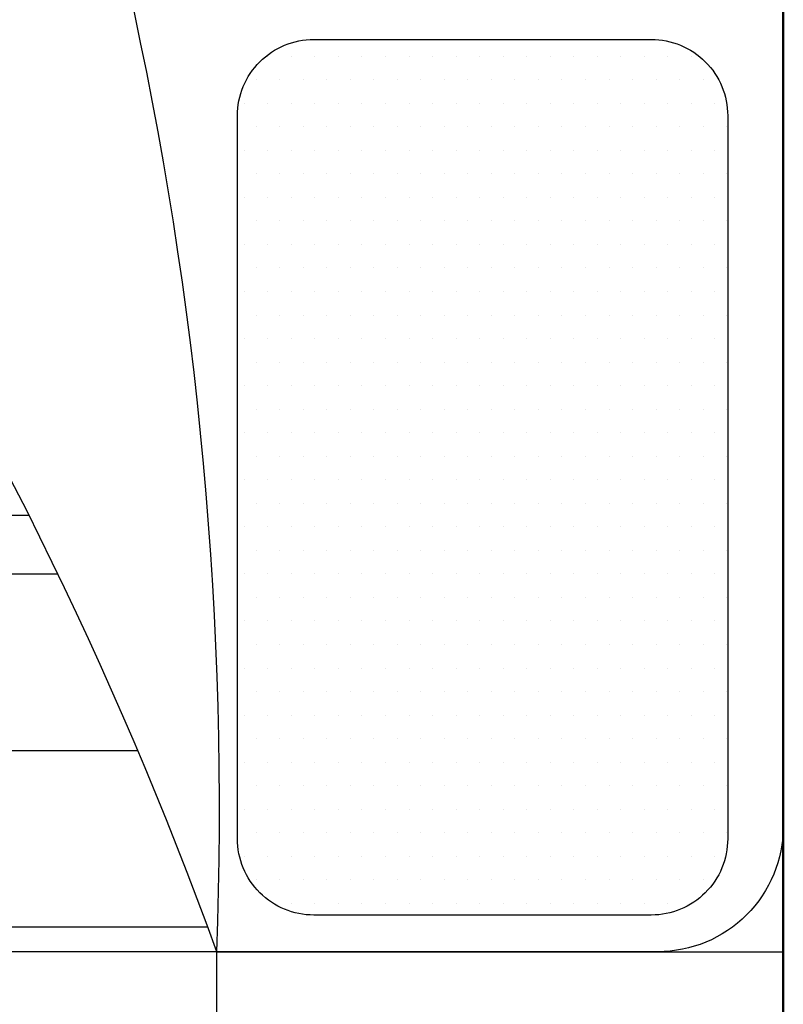
# Model space of a CAD drawing. Units: inches. Extents: x 3064 to 19385, y 846 to 15425.
# Tile 39 of 108: x 5302 to 5326, y 1028 to 1059. Entities that reach past the tile are written whole.
import ezdxf

# ---------------------------------------------------------------- set-up
doc = ezdxf.new("R2010")
doc.units = ezdxf.units.IN
doc.layers.add('A-FLOR-FIXT', color=9, linetype='Continuous', lineweight=18)
doc.layers.add('A-WALL', color=7, linetype='Continuous', lineweight=50)
doc.layers.add('BLOCK', color=6, linetype='Continuous')

# ---------------------------------------------------------------- blocks, each defined once
blk = doc.blocks.new('*X6')
at = {"color": 0}
for p, q in [((280.3125, 439.8862), (280.3125, 452.8965)), ((278.9062, 439.4824), (278.9062, 452.3385)), ((277.5, 439.4824), (277.5, 451.7019)), ((277.0312, 439.4824), (277.0312, 451.4714))]:
    blk.add_line(p, q, dxfattribs=at)
blk = doc.blocks.new('*X7')
at = {"color": 0}
for p, q in [((273.9375, 457.03125), (273.9375, 457.03125)), ((274.3125, 457.03125), (274.3125, 457.03125)), ((274.6875, 457.03125), (274.6875, 457.03125)), ((275.0625, 457.03125), (275.0625, 457.03125)), ((275.4375, 457.03125), (275.4375, 457.03125)), ((275.8125, 457.03125), (275.8125, 457.03125)), ((276.1875, 457.03125), (276.1875, 457.03125)), ((276.5625, 457.03125), (276.5625, 457.03125)), ((276.9375, 457.03125), (276.9375, 457.03125)), ((277.3125, 457.03125), (277.3125, 457.03125)), ((277.6875, 457.03125), (277.6875, 457.03125)), ((278.0625, 457.03125), (278.0625, 457.03125)), ((278.4375, 457.03125), (278.4375, 457.03125)), ((278.8125, 457.03125), (278.8125, 457.03125)), ((279.1875, 457.03125), (279.1875, 457.03125)), ((279.5625, 457.03125), (279.5625, 457.03125)), ((273.75, 456.9375), (273.75, 456.9375)), ((274.125, 456.9375), (274.125, 456.9375)), ((274.5, 456.9375), (274.5, 456.9375)), ((274.875, 456.9375), (274.875, 456.9375)), ((275.25, 456.9375), (275.25, 456.9375)), ((275.625, 456.9375), (275.625, 456.9375)), ((276, 456.9375), (276, 456.9375)), ((276.375, 456.9375), (276.375, 456.9375)), ((276.75, 456.9375), (276.75, 456.9375)), ((277.125, 456.9375), (277.125, 456.9375)), ((277.5, 456.9375), (277.5, 456.9375)), ((277.875, 456.9375), (277.875, 456.9375)), ((278.25, 456.9375), (278.25, 456.9375)), ((278.625, 456.9375), (278.625, 456.9375)), ((279, 456.9375), (279, 456.9375)), ((279.375, 456.9375), (279.375, 456.9375)), ((279.75, 456.9375), (279.75, 456.9375)), ((273.5625, 456.84375), (273.5625, 456.84375)), ((273.9375, 456.84375), (273.9375, 456.84375)), ((274.3125, 456.84375), (274.3125, 456.84375)), ((274.6875, 456.84375), (274.6875, 456.84375)), ((275.0625, 456.84375), (275.0625, 456.84375)), ((275.4375, 456.84375), (275.4375, 456.84375)), ((275.8125, 456.84375), (275.8125, 456.84375)), ((276.1875, 456.84375), (276.1875, 456.84375)), ((276.5625, 456.84375), (276.5625, 456.84375)), ((276.9375, 456.84375), (276.9375, 456.84375)), ((277.3125, 456.84375), (277.3125, 456.84375)), ((277.6875, 456.84375), (277.6875, 456.84375)), ((278.0625, 456.84375), (278.0625, 456.84375)), ((278.4375, 456.84375), (278.4375, 456.84375)), ((278.8125, 456.84375), (278.8125, 456.84375)), ((279.1875, 456.84375), (279.1875, 456.84375)), ((279.5625, 456.84375), (279.5625, 456.84375)), ((279.9375, 456.84375), (279.9375, 456.84375)), ((273.375, 456.75), (273.375, 456.75)), ((273.75, 456.75), (273.75, 456.75)), ((274.125, 456.75), (274.125, 456.75)), ((274.5, 456.75), (274.5, 456.75)), ((274.875, 456.75), (274.875, 456.75)), ((275.25, 456.75), (275.25, 456.75)), ((275.625, 456.75), (275.625, 456.75)), ((276, 456.75), (276, 456.75)), ((276.375, 456.75), (276.375, 456.75)), ((276.75, 456.75), (276.75, 456.75)), ((277.125, 456.75), (277.125, 456.75)), ((277.5, 456.75), (277.5, 456.75)), ((277.875, 456.75), (277.875, 456.75)), ((278.25, 456.75), (278.25, 456.75)), ((278.625, 456.75), (278.625, 456.75)), ((279, 456.75), (279, 456.75)), ((279.375, 456.75), (279.375, 456.75)), ((279.75, 456.75), (279.75, 456.75)), ((280.125, 456.75), (280.125, 456.75)), ((273.5625, 456.65625), (273.5625, 456.65625)), ((273.9375, 456.65625), (273.9375, 456.65625)), ((274.3125, 456.65625), (274.3125, 456.65625)), ((274.6875, 456.65625), (274.6875, 456.65625)), ((275.0625, 456.65625), (275.0625, 456.65625)), ((275.4375, 456.65625), (275.4375, 456.65625)), ((275.8125, 456.65625), (275.8125, 456.65625)), ((276.1875, 456.65625), (276.1875, 456.65625)), ((276.5625, 456.65625), (276.5625, 456.65625)), ((276.9375, 456.65625), (276.9375, 456.65625)), ((277.3125, 456.65625), (277.3125, 456.65625)), ((277.6875, 456.65625), (277.6875, 456.65625)), ((278.0625, 456.65625), (278.0625, 456.65625)), ((278.4375, 456.65625), (278.4375, 456.65625)), ((278.8125, 456.65625), (278.8125, 456.65625)), ((279.1875, 456.65625), (279.1875, 456.65625)), ((279.5625, 456.65625), (279.5625, 456.65625)), ((279.9375, 456.65625), (279.9375, 456.65625)), ((273.375, 456.5625), (273.375, 456.5625)), ((273.75, 456.5625), (273.75, 456.5625)), ((274.125, 456.5625), (274.125, 456.5625)), ((274.5, 456.5625), (274.5, 456.5625)), ((274.875, 456.5625), (274.875, 456.5625)), ((275.25, 456.5625), (275.25, 456.5625)), ((275.625, 456.5625), (275.625, 456.5625)), ((276, 456.5625), (276, 456.5625)), ((276.375, 456.5625), (276.375, 456.5625)), ((276.75, 456.5625), (276.75, 456.5625)), ((277.125, 456.5625), (277.125, 456.5625)), ((277.5, 456.5625), (277.5, 456.5625)), ((277.875, 456.5625), (277.875, 456.5625)), ((278.25, 456.5625), (278.25, 456.5625)), ((278.625, 456.5625), (278.625, 456.5625)), ((279, 456.5625), (279, 456.5625)), ((279.375, 456.5625), (279.375, 456.5625)), ((279.75, 456.5625), (279.75, 456.5625)), ((280.125, 456.5625), (280.125, 456.5625)), ((273.5625, 456.46875), (273.5625, 456.46875)), ((273.9375, 456.46875), (273.9375, 456.46875)), ((274.3125, 456.46875), (274.3125, 456.46875)), ((274.6875, 456.46875), (274.6875, 456.46875)), ((275.0625, 456.46875), (275.0625, 456.46875)), ((275.4375, 456.46875), (275.4375, 456.46875)), ((275.8125, 456.46875), (275.8125, 456.46875)), ((276.1875, 456.46875), (276.1875, 456.46875)), ((276.5625, 456.46875), (276.5625, 456.46875)), ((276.9375, 456.46875), (276.9375, 456.46875)), ((277.3125, 456.46875), (277.3125, 456.46875)), ((277.6875, 456.46875), (277.6875, 456.46875)), ((278.0625, 456.46875), (278.0625, 456.46875)), ((278.4375, 456.46875), (278.4375, 456.46875)), ((278.8125, 456.46875), (278.8125, 456.46875)), ((279.1875, 456.46875), (279.1875, 456.46875)), ((279.5625, 456.46875), (279.5625, 456.46875)), ((279.9375, 456.46875), (279.9375, 456.46875)), ((273.375, 456.375), (273.375, 456.375)), ((273.75, 456.375), (273.75, 456.375)), ((274.125, 456.375), (274.125, 456.375)), ((274.5, 456.375), (274.5, 456.375)), ((274.875, 456.375), (274.875, 456.375)), ((275.25, 456.375), (275.25, 456.375)), ((275.625, 456.375), (275.625, 456.375)), ((276, 456.375), (276, 456.375)), ((276.375, 456.375), (276.375, 456.375)), ((276.75, 456.375), (276.75, 456.375)), ((277.125, 456.375), (277.125, 456.375)), ((277.5, 456.375), (277.5, 456.375)), ((277.875, 456.375), (277.875, 456.375)), ((278.25, 456.375), (278.25, 456.375)), ((278.625, 456.375), (278.625, 456.375)), ((279, 456.375), (279, 456.375)), ((279.375, 456.375), (279.375, 456.375)), ((279.75, 456.375), (279.75, 456.375)), ((280.125, 456.375), (280.125, 456.375)), ((273.5625, 456.28125), (273.5625, 456.28125)), ((273.9375, 456.28125), (273.9375, 456.28125)), ((274.3125, 456.28125), (274.3125, 456.28125)), ((274.6875, 456.28125), (274.6875, 456.28125)), ((275.0625, 456.28125), (275.0625, 456.28125)), ((275.4375, 456.28125), (275.4375, 456.28125)), ((275.8125, 456.28125), (275.8125, 456.28125)), ((276.1875, 456.28125), (276.1875, 456.28125)), ((276.5625, 456.28125), (276.5625, 456.28125)), ((276.9375, 456.28125), (276.9375, 456.28125)), ((277.3125, 456.28125), (277.3125, 456.28125)), ((277.6875, 456.28125), (277.6875, 456.28125)), ((278.0625, 456.28125), (278.0625, 456.28125)), ((278.4375, 456.28125), (278.4375, 456.28125)), ((278.8125, 456.28125), (278.8125, 456.28125)), ((279.1875, 456.28125), (279.1875, 456.28125)), ((279.5625, 456.28125), (279.5625, 456.28125)), ((279.9375, 456.28125), (279.9375, 456.28125)), ((273.375, 456.1875), (273.375, 456.1875)), ((273.75, 456.1875), (273.75, 456.1875)), ((274.125, 456.1875), (274.125, 456.1875)), ((274.5, 456.1875), (274.5, 456.1875)), ((274.875, 456.1875), (274.875, 456.1875)), ((275.25, 456.1875), (275.25, 456.1875)), ((275.625, 456.1875), (275.625, 456.1875)), ((276, 456.1875), (276, 456.1875)), ((276.375, 456.1875), (276.375, 456.1875)), ((276.75, 456.1875), (276.75, 456.1875)), ((277.125, 456.1875), (277.125, 456.1875)), ((277.5, 456.1875), (277.5, 456.1875)), ((277.875, 456.1875), (277.875, 456.1875)), ((278.25, 456.1875), (278.25, 456.1875)), ((278.625, 456.1875), (278.625, 456.1875)), ((279, 456.1875), (279, 456.1875)), ((279.375, 456.1875), (279.375, 456.1875)), ((279.75, 456.1875), (279.75, 456.1875)), ((280.125, 456.1875), (280.125, 456.1875)), ((273.5625, 456.09375), (273.5625, 456.09375)), ((273.9375, 456.09375), (273.9375, 456.09375)), ((274.3125, 456.09375), (274.3125, 456.09375)), ((274.6875, 456.09375), (274.6875, 456.09375)), ((275.0625, 456.09375), (275.0625, 456.09375)), ((275.4375, 456.09375), (275.4375, 456.09375)), ((275.8125, 456.09375), (275.8125, 456.09375)), ((276.1875, 456.09375), (276.1875, 456.09375)), ((276.5625, 456.09375), (276.5625, 456.09375)), ((276.9375, 456.09375), (276.9375, 456.09375)), ((277.3125, 456.09375), (277.3125, 456.09375)), ((277.6875, 456.09375), (277.6875, 456.09375)), ((278.0625, 456.09375), (278.0625, 456.09375)), ((278.4375, 456.09375), (278.4375, 456.09375)), ((278.8125, 456.09375), (278.8125, 456.09375)), ((279.1875, 456.09375), (279.1875, 456.09375)), ((279.5625, 456.09375), (279.5625, 456.09375)), ((279.9375, 456.09375), (279.9375, 456.09375)), ((273.375, 456), (273.375, 456)), ((273.75, 456), (273.75, 456)), ((274.125, 456), (274.125, 456)), ((274.5, 456), (274.5, 456)), ((274.875, 456), (274.875, 456)), ((275.25, 456), (275.25, 456)), ((275.625, 456), (275.625, 456)), ((276, 456), (276, 456)), ((276.375, 456), (276.375, 456)), ((276.75, 456), (276.75, 456)), ((277.125, 456), (277.125, 456)), ((277.5, 456), (277.5, 456)), ((277.875, 456), (277.875, 456)), ((278.25, 456), (278.25, 456)), ((278.625, 456), (278.625, 456)), ((279, 456), (279, 456)), ((279.375, 456), (279.375, 456)), ((279.75, 456), (279.75, 456)), ((280.125, 456), (280.125, 456)), ((273.5625, 455.90625), (273.5625, 455.90625)), ((273.9375, 455.90625), (273.9375, 455.90625)), ((274.3125, 455.90625), (274.3125, 455.90625)), ((274.6875, 455.90625), (274.6875, 455.90625)), ((275.0625, 455.90625), (275.0625, 455.90625)), ((275.4375, 455.90625), (275.4375, 455.90625)), ((275.8125, 455.90625), (275.8125, 455.90625)), ((276.1875, 455.90625), (276.1875, 455.90625)), ((276.5625, 455.90625), (276.5625, 455.90625)), ((276.9375, 455.90625), (276.9375, 455.90625)), ((277.3125, 455.90625), (277.3125, 455.90625)), ((277.6875, 455.90625), (277.6875, 455.90625)), ((278.0625, 455.90625), (278.0625, 455.90625)), ((278.4375, 455.90625), (278.4375, 455.90625)), ((278.8125, 455.90625), (278.8125, 455.90625)), ((279.1875, 455.90625), (279.1875, 455.90625)), ((279.5625, 455.90625), (279.5625, 455.90625)), ((279.9375, 455.90625), (279.9375, 455.90625)), ((273.375, 455.8125), (273.375, 455.8125)), ((273.75, 455.8125), (273.75, 455.8125)), ((274.125, 455.8125), (274.125, 455.8125)), ((274.5, 455.8125), (274.5, 455.8125)), ((274.875, 455.8125), (274.875, 455.8125)), ((275.25, 455.8125), (275.25, 455.8125)), ((275.625, 455.8125), (275.625, 455.8125)), ((276, 455.8125), (276, 455.8125)), ((276.375, 455.8125), (276.375, 455.8125)), ((276.75, 455.8125), (276.75, 455.8125)), ((277.125, 455.8125), (277.125, 455.8125)), ((277.5, 455.8125), (277.5, 455.8125)), ((277.875, 455.8125), (277.875, 455.8125)), ((278.25, 455.8125), (278.25, 455.8125)), ((278.625, 455.8125), (278.625, 455.8125)), ((279, 455.8125), (279, 455.8125)), ((279.375, 455.8125), (279.375, 455.8125)), ((279.75, 455.8125), (279.75, 455.8125)), ((280.125, 455.8125), (280.125, 455.8125)), ((273.5625, 455.71875), (273.5625, 455.71875)), ((273.9375, 455.71875), (273.9375, 455.71875)), ((274.3125, 455.71875), (274.3125, 455.71875)), ((274.6875, 455.71875), (274.6875, 455.71875)), ((275.0625, 455.71875), (275.0625, 455.71875)), ((275.4375, 455.71875), (275.4375, 455.71875)), ((275.8125, 455.71875), (275.8125, 455.71875)), ((276.1875, 455.71875), (276.1875, 455.71875)), ((276.5625, 455.71875), (276.5625, 455.71875)), ((276.9375, 455.71875), (276.9375, 455.71875)), ((277.3125, 455.71875), (277.3125, 455.71875)), ((277.6875, 455.71875), (277.6875, 455.71875)), ((278.0625, 455.71875), (278.0625, 455.71875)), ((278.4375, 455.71875), (278.4375, 455.71875)), ((278.8125, 455.71875), (278.8125, 455.71875)), ((279.1875, 455.71875), (279.1875, 455.71875)), ((279.5625, 455.71875), (279.5625, 455.71875)), ((279.9375, 455.71875), (279.9375, 455.71875)), ((273.375, 455.625), (273.375, 455.625)), ((273.75, 455.625), (273.75, 455.625)), ((274.125, 455.625), (274.125, 455.625)), ((274.5, 455.625), (274.5, 455.625)), ((274.875, 455.625), (274.875, 455.625)), ((275.25, 455.625), (275.25, 455.625)), ((275.625, 455.625), (275.625, 455.625)), ((276, 455.625), (276, 455.625)), ((276.375, 455.625), (276.375, 455.625)), ((276.75, 455.625), (276.75, 455.625)), ((277.125, 455.625), (277.125, 455.625)), ((277.5, 455.625), (277.5, 455.625)), ((277.875, 455.625), (277.875, 455.625)), ((278.25, 455.625), (278.25, 455.625)), ((278.625, 455.625), (278.625, 455.625)), ((279, 455.625), (279, 455.625)), ((279.375, 455.625), (279.375, 455.625)), ((279.75, 455.625), (279.75, 455.625)), ((280.125, 455.625), (280.125, 455.625)), ((273.5625, 455.53125), (273.5625, 455.53125)), ((273.9375, 455.53125), (273.9375, 455.53125)), ((274.3125, 455.53125), (274.3125, 455.53125)), ((274.6875, 455.53125), (274.6875, 455.53125)), ((275.0625, 455.53125), (275.0625, 455.53125)), ((275.4375, 455.53125), (275.4375, 455.53125)), ((275.8125, 455.53125), (275.8125, 455.53125)), ((276.1875, 455.53125), (276.1875, 455.53125)), ((276.5625, 455.53125), (276.5625, 455.53125)), ((276.9375, 455.53125), (276.9375, 455.53125)), ((277.3125, 455.53125), (277.3125, 455.53125)), ((277.6875, 455.53125), (277.6875, 455.53125)), ((278.0625, 455.53125), (278.0625, 455.53125)), ((278.4375, 455.53125), (278.4375, 455.53125)), ((278.8125, 455.53125), (278.8125, 455.53125)), ((279.1875, 455.53125), (279.1875, 455.53125)), ((279.5625, 455.53125), (279.5625, 455.53125)), ((279.9375, 455.53125), (279.9375, 455.53125)), ((273.375, 455.4375), (273.375, 455.4375)), ((273.75, 455.4375), (273.75, 455.4375)), ((274.125, 455.4375), (274.125, 455.4375)), ((274.5, 455.4375), (274.5, 455.4375)), ((274.875, 455.4375), (274.875, 455.4375)), ((275.25, 455.4375), (275.25, 455.4375)), ((275.625, 455.4375), (275.625, 455.4375)), ((276, 455.4375), (276, 455.4375)), ((276.375, 455.4375), (276.375, 455.4375)), ((276.75, 455.4375), (276.75, 455.4375)), ((277.125, 455.4375), (277.125, 455.4375)), ((277.5, 455.4375), (277.5, 455.4375)), ((277.875, 455.4375), (277.875, 455.4375)), ((278.25, 455.4375), (278.25, 455.4375)), ((278.625, 455.4375), (278.625, 455.4375)), ((279, 455.4375), (279, 455.4375)), ((279.375, 455.4375), (279.375, 455.4375)), ((279.75, 455.4375), (279.75, 455.4375)), ((280.125, 455.4375), (280.125, 455.4375)), ((273.5625, 455.34375), (273.5625, 455.34375)), ((273.9375, 455.34375), (273.9375, 455.34375)), ((274.3125, 455.34375), (274.3125, 455.34375)), ((274.6875, 455.34375), (274.6875, 455.34375)), ((275.0625, 455.34375), (275.0625, 455.34375)), ((275.4375, 455.34375), (275.4375, 455.34375)), ((275.8125, 455.34375), (275.8125, 455.34375)), ((276.1875, 455.34375), (276.1875, 455.34375)), ((276.5625, 455.34375), (276.5625, 455.34375)), ((276.9375, 455.34375), (276.9375, 455.34375)), ((277.3125, 455.34375), (277.3125, 455.34375)), ((277.6875, 455.34375), (277.6875, 455.34375)), ((278.0625, 455.34375), (278.0625, 455.34375)), ((278.4375, 455.34375), (278.4375, 455.34375)), ((278.8125, 455.34375), (278.8125, 455.34375)), ((279.1875, 455.34375), (279.1875, 455.34375)), ((279.5625, 455.34375), (279.5625, 455.34375)), ((279.9375, 455.34375), (279.9375, 455.34375)), ((273.375, 455.25), (273.375, 455.25)), ((273.75, 455.25), (273.75, 455.25)), ((274.125, 455.25), (274.125, 455.25)), ((274.5, 455.25), (274.5, 455.25)), ((274.875, 455.25), (274.875, 455.25)), ((275.25, 455.25), (275.25, 455.25)), ((275.625, 455.25), (275.625, 455.25)), ((276, 455.25), (276, 455.25)), ((276.375, 455.25), (276.375, 455.25)), ((276.75, 455.25), (276.75, 455.25)), ((277.125, 455.25), (277.125, 455.25)), ((277.5, 455.25), (277.5, 455.25)), ((277.875, 455.25), (277.875, 455.25)), ((278.25, 455.25), (278.25, 455.25)), ((278.625, 455.25), (278.625, 455.25)), ((279, 455.25), (279, 455.25)), ((279.375, 455.25), (279.375, 455.25)), ((279.75, 455.25), (279.75, 455.25)), ((280.125, 455.25), (280.125, 455.25)), ((273.5625, 455.15625), (273.5625, 455.15625)), ((273.9375, 455.15625), (273.9375, 455.15625)), ((274.3125, 455.15625), (274.3125, 455.15625)), ((274.6875, 455.15625), (274.6875, 455.15625)), ((275.0625, 455.15625), (275.0625, 455.15625)), ((275.4375, 455.15625), (275.4375, 455.15625)), ((275.8125, 455.15625), (275.8125, 455.15625)), ((276.1875, 455.15625), (276.1875, 455.15625)), ((276.5625, 455.15625), (276.5625, 455.15625)), ((276.9375, 455.15625), (276.9375, 455.15625)), ((277.3125, 455.15625), (277.3125, 455.15625)), ((277.6875, 455.15625), (277.6875, 455.15625)), ((278.0625, 455.15625), (278.0625, 455.15625)), ((278.4375, 455.15625), (278.4375, 455.15625)), ((278.8125, 455.15625), (278.8125, 455.15625)), ((279.1875, 455.15625), (279.1875, 455.15625)), ((279.5625, 455.15625), (279.5625, 455.15625)), ((279.9375, 455.15625), (279.9375, 455.15625)), ((273.375, 455.0625), (273.375, 455.0625)), ((273.75, 455.0625), (273.75, 455.0625)), ((274.125, 455.0625), (274.125, 455.0625)), ((274.5, 455.0625), (274.5, 455.0625)), ((274.875, 455.0625), (274.875, 455.0625)), ((275.25, 455.0625), (275.25, 455.0625)), ((275.625, 455.0625), (275.625, 455.0625)), ((276, 455.0625), (276, 455.0625)), ((276.375, 455.0625), (276.375, 455.0625)), ((276.75, 455.0625), (276.75, 455.0625)), ((277.125, 455.0625), (277.125, 455.0625)), ((277.5, 455.0625), (277.5, 455.0625)), ((277.875, 455.0625), (277.875, 455.0625)), ((278.25, 455.0625), (278.25, 455.0625)), ((278.625, 455.0625), (278.625, 455.0625)), ((279, 455.0625), (279, 455.0625)), ((279.375, 455.0625), (279.375, 455.0625)), ((279.75, 455.0625), (279.75, 455.0625)), ((280.125, 455.0625), (280.125, 455.0625)), ((273.5625, 454.96875), (273.5625, 454.96875)), ((273.9375, 454.96875), (273.9375, 454.96875)), ((274.3125, 454.96875), (274.3125, 454.96875)), ((274.6875, 454.96875), (274.6875, 454.96875)), ((275.0625, 454.96875), (275.0625, 454.96875)), ((275.4375, 454.96875), (275.4375, 454.96875)), ((275.8125, 454.96875), (275.8125, 454.96875)), ((276.1875, 454.96875), (276.1875, 454.96875)), ((276.5625, 454.96875), (276.5625, 454.96875)), ((276.9375, 454.96875), (276.9375, 454.96875)), ((277.3125, 454.96875), (277.3125, 454.96875)), ((277.6875, 454.96875), (277.6875, 454.96875)), ((278.0625, 454.96875), (278.0625, 454.96875)), ((278.4375, 454.96875), (278.4375, 454.96875)), ((278.8125, 454.96875), (278.8125, 454.96875)), ((279.1875, 454.96875), (279.1875, 454.96875)), ((279.5625, 454.96875), (279.5625, 454.96875)), ((279.9375, 454.96875), (279.9375, 454.96875)), ((273.375, 454.875), (273.375, 454.875)), ((273.75, 454.875), (273.75, 454.875)), ((274.125, 454.875), (274.125, 454.875)), ((274.5, 454.875), (274.5, 454.875)), ((274.875, 454.875), (274.875, 454.875)), ((275.25, 454.875), (275.25, 454.875)), ((275.625, 454.875), (275.625, 454.875)), ((276, 454.875), (276, 454.875)), ((276.375, 454.875), (276.375, 454.875)), ((276.75, 454.875), (276.75, 454.875)), ((277.125, 454.875), (277.125, 454.875)), ((277.5, 454.875), (277.5, 454.875)), ((277.875, 454.875), (277.875, 454.875)), ((278.25, 454.875), (278.25, 454.875)), ((278.625, 454.875), (278.625, 454.875)), ((279, 454.875), (279, 454.875)), ((279.375, 454.875), (279.375, 454.875)), ((279.75, 454.875), (279.75, 454.875)), ((280.125, 454.875), (280.125, 454.875)), ((273.5625, 454.78125), (273.5625, 454.78125)), ((273.9375, 454.78125), (273.9375, 454.78125)), ((274.3125, 454.78125), (274.3125, 454.78125)), ((274.6875, 454.78125), (274.6875, 454.78125)), ((275.0625, 454.78125), (275.0625, 454.78125)), ((275.4375, 454.78125), (275.4375, 454.78125)), ((275.8125, 454.78125), (275.8125, 454.78125)), ((276.1875, 454.78125), (276.1875, 454.78125)), ((276.5625, 454.78125), (276.5625, 454.78125)), ((276.9375, 454.78125), (276.9375, 454.78125)), ((277.3125, 454.78125), (277.3125, 454.78125)), ((277.6875, 454.78125), (277.6875, 454.78125)), ((278.0625, 454.78125), (278.0625, 454.78125)), ((278.4375, 454.78125), (278.4375, 454.78125)), ((278.8125, 454.78125), (278.8125, 454.78125)), ((279.1875, 454.78125), (279.1875, 454.78125)), ((279.5625, 454.78125), (279.5625, 454.78125)), ((279.9375, 454.78125), (279.9375, 454.78125)), ((273.375, 454.6875), (273.375, 454.6875)), ((273.75, 454.6875), (273.75, 454.6875)), ((274.125, 454.6875), (274.125, 454.6875)), ((274.5, 454.6875), (274.5, 454.6875)), ((274.875, 454.6875), (274.875, 454.6875)), ((275.25, 454.6875), (275.25, 454.6875)), ((275.625, 454.6875), (275.625, 454.6875)), ((276, 454.6875), (276, 454.6875)), ((276.375, 454.6875), (276.375, 454.6875)), ((276.75, 454.6875), (276.75, 454.6875)), ((277.125, 454.6875), (277.125, 454.6875)), ((277.5, 454.6875), (277.5, 454.6875)), ((277.875, 454.6875), (277.875, 454.6875)), ((278.25, 454.6875), (278.25, 454.6875)), ((278.625, 454.6875), (278.625, 454.6875)), ((279, 454.6875), (279, 454.6875)), ((279.375, 454.6875), (279.375, 454.6875)), ((279.75, 454.6875), (279.75, 454.6875)), ((280.125, 454.6875), (280.125, 454.6875)), ((273.5625, 454.59375), (273.5625, 454.59375)), ((273.9375, 454.59375), (273.9375, 454.59375)), ((274.3125, 454.59375), (274.3125, 454.59375)), ((274.6875, 454.59375), (274.6875, 454.59375)), ((275.0625, 454.59375), (275.0625, 454.59375)), ((275.4375, 454.59375), (275.4375, 454.59375)), ((275.8125, 454.59375), (275.8125, 454.59375)), ((276.1875, 454.59375), (276.1875, 454.59375)), ((276.5625, 454.59375), (276.5625, 454.59375)), ((276.9375, 454.59375), (276.9375, 454.59375)), ((277.3125, 454.59375), (277.3125, 454.59375)), ((277.6875, 454.59375), (277.6875, 454.59375)), ((278.0625, 454.59375), (278.0625, 454.59375)), ((278.4375, 454.59375), (278.4375, 454.59375)), ((278.8125, 454.59375), (278.8125, 454.59375)), ((279.1875, 454.59375), (279.1875, 454.59375)), ((279.5625, 454.59375), (279.5625, 454.59375)), ((279.9375, 454.59375), (279.9375, 454.59375)), ((273.375, 454.5), (273.375, 454.5)), ((273.75, 454.5), (273.75, 454.5)), ((274.125, 454.5), (274.125, 454.5)), ((274.5, 454.5), (274.5, 454.5)), ((274.875, 454.5), (274.875, 454.5)), ((275.25, 454.5), (275.25, 454.5)), ((275.625, 454.5), (275.625, 454.5)), ((276, 454.5), (276, 454.5)), ((276.375, 454.5), (276.375, 454.5)), ((276.75, 454.5), (276.75, 454.5)), ((277.125, 454.5), (277.125, 454.5)), ((277.5, 454.5), (277.5, 454.5)), ((277.875, 454.5), (277.875, 454.5)), ((278.25, 454.5), (278.25, 454.5)), ((278.625, 454.5), (278.625, 454.5)), ((279, 454.5), (279, 454.5)), ((279.375, 454.5), (279.375, 454.5)), ((279.75, 454.5), (279.75, 454.5)), ((280.125, 454.5), (280.125, 454.5)), ((273.5625, 454.40625), (273.5625, 454.40625)), ((273.9375, 454.40625), (273.9375, 454.40625)), ((274.3125, 454.40625), (274.3125, 454.40625)), ((274.6875, 454.40625), (274.6875, 454.40625)), ((275.0625, 454.40625), (275.0625, 454.40625)), ((275.4375, 454.40625), (275.4375, 454.40625)), ((275.8125, 454.40625), (275.8125, 454.40625)), ((276.1875, 454.40625), (276.1875, 454.40625)), ((276.5625, 454.40625), (276.5625, 454.40625)), ((276.9375, 454.40625), (276.9375, 454.40625)), ((277.3125, 454.40625), (277.3125, 454.40625)), ((277.6875, 454.40625), (277.6875, 454.40625)), ((278.0625, 454.40625), (278.0625, 454.40625)), ((278.4375, 454.40625), (278.4375, 454.40625)), ((278.8125, 454.40625), (278.8125, 454.40625)), ((279.1875, 454.40625), (279.1875, 454.40625)), ((279.5625, 454.40625), (279.5625, 454.40625)), ((279.9375, 454.40625), (279.9375, 454.40625)), ((273.375, 454.3125), (273.375, 454.3125)), ((273.75, 454.3125), (273.75, 454.3125)), ((274.125, 454.3125), (274.125, 454.3125)), ((274.5, 454.3125), (274.5, 454.3125)), ((274.875, 454.3125), (274.875, 454.3125)), ((275.25, 454.3125), (275.25, 454.3125)), ((275.625, 454.3125), (275.625, 454.3125)), ((276, 454.3125), (276, 454.3125)), ((276.375, 454.3125), (276.375, 454.3125)), ((276.75, 454.3125), (276.75, 454.3125)), ((277.125, 454.3125), (277.125, 454.3125)), ((277.5, 454.3125), (277.5, 454.3125)), ((277.875, 454.3125), (277.875, 454.3125)), ((278.25, 454.3125), (278.25, 454.3125)), ((278.625, 454.3125), (278.625, 454.3125)), ((279, 454.3125), (279, 454.3125)), ((279.375, 454.3125), (279.375, 454.3125)), ((279.75, 454.3125), (279.75, 454.3125)), ((280.125, 454.3125), (280.125, 454.3125)), ((273.5625, 454.21875), (273.5625, 454.21875)), ((273.9375, 454.21875), (273.9375, 454.21875)), ((274.3125, 454.21875), (274.3125, 454.21875)), ((274.6875, 454.21875), (274.6875, 454.21875)), ((275.0625, 454.21875), (275.0625, 454.21875)), ((275.4375, 454.21875), (275.4375, 454.21875)), ((275.8125, 454.21875), (275.8125, 454.21875)), ((276.1875, 454.21875), (276.1875, 454.21875)), ((276.5625, 454.21875), (276.5625, 454.21875)), ((276.9375, 454.21875), (276.9375, 454.21875)), ((277.3125, 454.21875), (277.3125, 454.21875)), ((277.6875, 454.21875), (277.6875, 454.21875)), ((278.0625, 454.21875), (278.0625, 454.21875)), ((278.4375, 454.21875), (278.4375, 454.21875)), ((278.8125, 454.21875), (278.8125, 454.21875)), ((279.1875, 454.21875), (279.1875, 454.21875)), ((279.5625, 454.21875), (279.5625, 454.21875)), ((279.9375, 454.21875), (279.9375, 454.21875)), ((273.375, 454.125), (273.375, 454.125)), ((273.75, 454.125), (273.75, 454.125)), ((274.125, 454.125), (274.125, 454.125)), ((274.5, 454.125), (274.5, 454.125)), ((274.875, 454.125), (274.875, 454.125)), ((275.25, 454.125), (275.25, 454.125)), ((275.625, 454.125), (275.625, 454.125)), ((276, 454.125), (276, 454.125)), ((276.375, 454.125), (276.375, 454.125)), ((276.75, 454.125), (276.75, 454.125)), ((277.125, 454.125), (277.125, 454.125)), ((277.5, 454.125), (277.5, 454.125)), ((277.875, 454.125), (277.875, 454.125)), ((278.25, 454.125), (278.25, 454.125)), ((278.625, 454.125), (278.625, 454.125)), ((279, 454.125), (279, 454.125)), ((279.375, 454.125), (279.375, 454.125)), ((279.75, 454.125), (279.75, 454.125)), ((280.125, 454.125), (280.125, 454.125)), ((273.5625, 454.03125), (273.5625, 454.03125)), ((273.9375, 454.03125), (273.9375, 454.03125)), ((274.3125, 454.03125), (274.3125, 454.03125)), ((274.6875, 454.03125), (274.6875, 454.03125)), ((275.0625, 454.03125), (275.0625, 454.03125)), ((275.4375, 454.03125), (275.4375, 454.03125)), ((275.8125, 454.03125), (275.8125, 454.03125)), ((276.1875, 454.03125), (276.1875, 454.03125)), ((276.5625, 454.03125), (276.5625, 454.03125)), ((276.9375, 454.03125), (276.9375, 454.03125)), ((277.3125, 454.03125), (277.3125, 454.03125)), ((277.6875, 454.03125), (277.6875, 454.03125)), ((278.0625, 454.03125), (278.0625, 454.03125)), ((278.4375, 454.03125), (278.4375, 454.03125)), ((278.8125, 454.03125), (278.8125, 454.03125)), ((279.1875, 454.03125), (279.1875, 454.03125)), ((279.5625, 454.03125), (279.5625, 454.03125)), ((279.9375, 454.03125), (279.9375, 454.03125)), ((273.375, 453.9375), (273.375, 453.9375)), ((273.75, 453.9375), (273.75, 453.9375)), ((274.125, 453.9375), (274.125, 453.9375)), ((274.5, 453.9375), (274.5, 453.9375)), ((274.875, 453.9375), (274.875, 453.9375)), ((275.25, 453.9375), (275.25, 453.9375)), ((275.625, 453.9375), (275.625, 453.9375)), ((276, 453.9375), (276, 453.9375)), ((276.375, 453.9375), (276.375, 453.9375)), ((276.75, 453.9375), (276.75, 453.9375)), ((277.125, 453.9375), (277.125, 453.9375)), ((277.5, 453.9375), (277.5, 453.9375)), ((277.875, 453.9375), (277.875, 453.9375)), ((278.25, 453.9375), (278.25, 453.9375)), ((278.625, 453.9375), (278.625, 453.9375)), ((279, 453.9375), (279, 453.9375)), ((279.375, 453.9375), (279.375, 453.9375)), ((279.75, 453.9375), (279.75, 453.9375)), ((280.125, 453.9375), (280.125, 453.9375)), ((273.5625, 453.84375), (273.5625, 453.84375)), ((273.9375, 453.84375), (273.9375, 453.84375)), ((274.3125, 453.84375), (274.3125, 453.84375)), ((274.6875, 453.84375), (274.6875, 453.84375)), ((275.0625, 453.84375), (275.0625, 453.84375)), ((275.4375, 453.84375), (275.4375, 453.84375)), ((275.8125, 453.84375), (275.8125, 453.84375)), ((276.1875, 453.84375), (276.1875, 453.84375)), ((276.5625, 453.84375), (276.5625, 453.84375)), ((276.9375, 453.84375), (276.9375, 453.84375)), ((277.3125, 453.84375), (277.3125, 453.84375)), ((277.6875, 453.84375), (277.6875, 453.84375)), ((278.0625, 453.84375), (278.0625, 453.84375)), ((278.4375, 453.84375), (278.4375, 453.84375)), ((278.8125, 453.84375), (278.8125, 453.84375)), ((279.1875, 453.84375), (279.1875, 453.84375)), ((279.5625, 453.84375), (279.5625, 453.84375)), ((279.9375, 453.84375), (279.9375, 453.84375)), ((273.375, 453.75), (273.375, 453.75)), ((273.75, 453.75), (273.75, 453.75)), ((274.125, 453.75), (274.125, 453.75)), ((274.5, 453.75), (274.5, 453.75)), ((274.875, 453.75), (274.875, 453.75)), ((275.25, 453.75), (275.25, 453.75)), ((275.625, 453.75), (275.625, 453.75)), ((276, 453.75), (276, 453.75)), ((276.375, 453.75), (276.375, 453.75)), ((276.75, 453.75), (276.75, 453.75)), ((277.125, 453.75), (277.125, 453.75)), ((277.5, 453.75), (277.5, 453.75)), ((277.875, 453.75), (277.875, 453.75)), ((278.25, 453.75), (278.25, 453.75)), ((278.625, 453.75), (278.625, 453.75)), ((279, 453.75), (279, 453.75)), ((279.375, 453.75), (279.375, 453.75)), ((279.75, 453.75), (279.75, 453.75)), ((280.125, 453.75), (280.125, 453.75)), ((273.5625, 453.65625), (273.5625, 453.65625)), ((273.9375, 453.65625), (273.9375, 453.65625)), ((274.3125, 453.65625), (274.3125, 453.65625)), ((274.6875, 453.65625), (274.6875, 453.65625)), ((275.0625, 453.65625), (275.0625, 453.65625)), ((275.4375, 453.65625), (275.4375, 453.65625)), ((275.8125, 453.65625), (275.8125, 453.65625)), ((276.1875, 453.65625), (276.1875, 453.65625)), ((276.5625, 453.65625), (276.5625, 453.65625)), ((276.9375, 453.65625), (276.9375, 453.65625)), ((277.3125, 453.65625), (277.3125, 453.65625)), ((277.6875, 453.65625), (277.6875, 453.65625)), ((278.0625, 453.65625), (278.0625, 453.65625)), ((278.4375, 453.65625), (278.4375, 453.65625)), ((278.8125, 453.65625), (278.8125, 453.65625)), ((279.1875, 453.65625), (279.1875, 453.65625)), ((279.5625, 453.65625), (279.5625, 453.65625)), ((279.9375, 453.65625), (279.9375, 453.65625)), ((273.375, 453.5625), (273.375, 453.5625)), ((273.75, 453.5625), (273.75, 453.5625)), ((274.125, 453.5625), (274.125, 453.5625)), ((274.5, 453.5625), (274.5, 453.5625)), ((274.875, 453.5625), (274.875, 453.5625)), ((275.25, 453.5625), (275.25, 453.5625)), ((275.625, 453.5625), (275.625, 453.5625)), ((276, 453.5625), (276, 453.5625)), ((276.375, 453.5625), (276.375, 453.5625)), ((276.75, 453.5625), (276.75, 453.5625)), ((277.125, 453.5625), (277.125, 453.5625)), ((277.5, 453.5625), (277.5, 453.5625)), ((277.875, 453.5625), (277.875, 453.5625)), ((278.25, 453.5625), (278.25, 453.5625)), ((278.625, 453.5625), (278.625, 453.5625)), ((279, 453.5625), (279, 453.5625)), ((279.375, 453.5625), (279.375, 453.5625)), ((279.75, 453.5625), (279.75, 453.5625)), ((280.125, 453.5625), (280.125, 453.5625)), ((273.5625, 453.46875), (273.5625, 453.46875)), ((273.9375, 453.46875), (273.9375, 453.46875)), ((274.3125, 453.46875), (274.3125, 453.46875)), ((274.6875, 453.46875), (274.6875, 453.46875)), ((275.0625, 453.46875), (275.0625, 453.46875)), ((275.4375, 453.46875), (275.4375, 453.46875)), ((275.8125, 453.46875), (275.8125, 453.46875)), ((276.1875, 453.46875), (276.1875, 453.46875)), ((276.5625, 453.46875), (276.5625, 453.46875)), ((276.9375, 453.46875), (276.9375, 453.46875)), ((277.3125, 453.46875), (277.3125, 453.46875)), ((277.6875, 453.46875), (277.6875, 453.46875)), ((278.0625, 453.46875), (278.0625, 453.46875)), ((278.4375, 453.46875), (278.4375, 453.46875)), ((278.8125, 453.46875), (278.8125, 453.46875)), ((279.1875, 453.46875), (279.1875, 453.46875)), ((279.5625, 453.46875), (279.5625, 453.46875)), ((279.9375, 453.46875), (279.9375, 453.46875)), ((273.375, 453.375), (273.375, 453.375)), ((273.75, 453.375), (273.75, 453.375)), ((274.125, 453.375), (274.125, 453.375)), ((274.5, 453.375), (274.5, 453.375)), ((274.875, 453.375), (274.875, 453.375)), ((275.25, 453.375), (275.25, 453.375)), ((275.625, 453.375), (275.625, 453.375)), ((276, 453.375), (276, 453.375)), ((276.375, 453.375), (276.375, 453.375)), ((276.75, 453.375), (276.75, 453.375)), ((277.125, 453.375), (277.125, 453.375)), ((277.5, 453.375), (277.5, 453.375)), ((277.875, 453.375), (277.875, 453.375)), ((278.25, 453.375), (278.25, 453.375)), ((278.625, 453.375), (278.625, 453.375)), ((279, 453.375), (279, 453.375)), ((279.375, 453.375), (279.375, 453.375)), ((279.75, 453.375), (279.75, 453.375)), ((273.5625, 453.28125), (273.5625, 453.28125)), ((273.9375, 453.28125), (273.9375, 453.28125)), ((274.3125, 453.28125), (274.3125, 453.28125)), ((274.6875, 453.28125), (274.6875, 453.28125)), ((275.0625, 453.28125), (275.0625, 453.28125)), ((275.4375, 453.28125), (275.4375, 453.28125)), ((275.8125, 453.28125), (275.8125, 453.28125)), ((276.1875, 453.28125), (276.1875, 453.28125)), ((276.5625, 453.28125), (276.5625, 453.28125)), ((276.9375, 453.28125), (276.9375, 453.28125)), ((277.3125, 453.28125), (277.3125, 453.28125)), ((277.6875, 453.28125), (277.6875, 453.28125)), ((278.0625, 453.28125), (278.0625, 453.28125)), ((278.4375, 453.28125), (278.4375, 453.28125)), ((278.8125, 453.28125), (278.8125, 453.28125)), ((279.1875, 453.28125), (279.1875, 453.28125)), ((279.5625, 453.28125), (279.5625, 453.28125)), ((279.9375, 453.28125), (279.9375, 453.28125)), ((273.75, 453.1875), (273.75, 453.1875)), ((274.125, 453.1875), (274.125, 453.1875)), ((274.5, 453.1875), (274.5, 453.1875)), ((274.875, 453.1875), (274.875, 453.1875)), ((275.25, 453.1875), (275.25, 453.1875)), ((275.625, 453.1875), (275.625, 453.1875)), ((276, 453.1875), (276, 453.1875)), ((276.375, 453.1875), (276.375, 453.1875)), ((276.75, 453.1875), (276.75, 453.1875)), ((277.125, 453.1875), (277.125, 453.1875)), ((277.5, 453.1875), (277.5, 453.1875)), ((277.875, 453.1875), (277.875, 453.1875)), ((278.25, 453.1875), (278.25, 453.1875)), ((278.625, 453.1875), (278.625, 453.1875)), ((279, 453.1875), (279, 453.1875)), ((279.375, 453.1875), (279.375, 453.1875)), ((279.75, 453.1875), (279.75, 453.1875))]:
    blk.add_line(p, q, dxfattribs=at)
blk = doc.blocks.new('A$C52E67D0D')
at = {"layer": 'BLOCK'}
for points in [[(1901, 0), (601, 0, -0.414214), (501, 100), (501, 1700, -0.414214), (601, 1800), (1901, 1800, -0.414214), (2001, 1700), (2001, 100, -0.414214)], [(1910.98, 1365.08), (1335.04, 1365.08, -0.414214), (1274.19, 1425.93), (1274.19, 1694.83, -0.414214), (1335.04, 1755.67), (1910.98, 1755.67, -0.414214), (1971.82, 1694.83), (1971.82, 1425.93, -0.414214)]]:
    blk.add_lwpolyline(points, format="xyb", close=True, dxfattribs=at)
blk.add_lwpolyline([(2001, 1348.63), (2001, 1799.63), (2502, 1799.63), (2502, 1348.63)], close=True, dxfattribs=at)
for centre, radius, start, end in [((1888.63, -1664.54), 3015.26, 87.86419, 117.40011), ((3101.01, -1685.8), 3227.66, 109.92605, 135.39771)]:
    blk.add_arc(centre, radius, start, end, dxfattribs=at)
at = {"layer": 'BLOCK', "xscale": 100, "yscale": 100, "zscale": 100}
for name in ['*X7', '*X6']:
    blk.add_blockref(name, (-26049.96, -43948.24), dxfattribs=at)

msp = doc.modelspace()

# ---------------------------------------------------------------- linework, layer by layer
at = {"layer": 'A-WALL'}
msp.add_line((5326.017, 1140.096), (5326.017, 978.096), dxfattribs=at)

# ---------------------------------------------------------------- block references
at = {"layer": 'A-FLOR-FIXT', "xscale": 0.039370099999992, "yscale": 0.039370099999992, "zscale": 0.039370099999992, "rotation": 270}
msp.add_blockref('A$C52E67D0D', (5255.151, 1108.348), dxfattribs=at)

doc.saveas('drawing.dxf')
